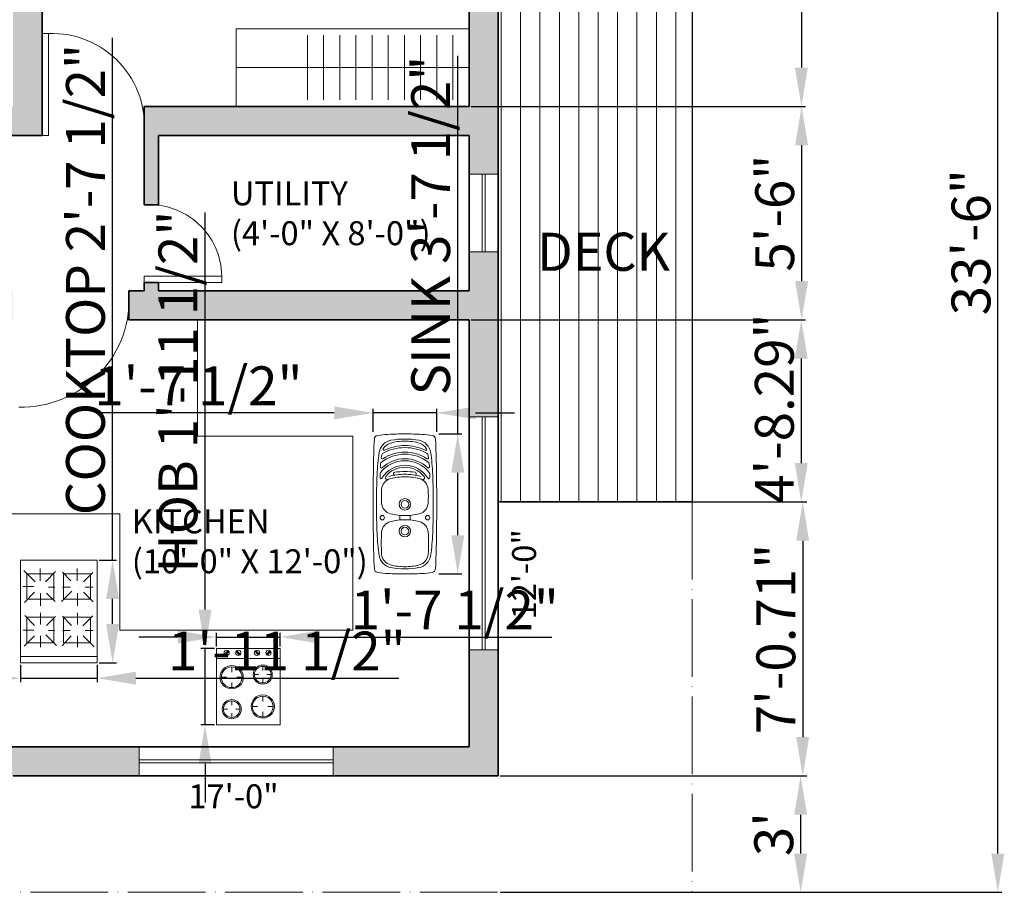
# Model space of a CAD drawing. Units: inches. Extents: x 2364 to 7426, y 1289 to 11972.
# Tile 4 of 6: x 2923 to 3228, y 1362 to 1631. Entities that reach past the tile are written whole.
import ezdxf

# ---------------------------------------------------------------- set-up
doc = ezdxf.new("R2010")
doc.units = ezdxf.units.IN
doc.linetypes.add('ACAD_ISO04W100', pattern=[30, 24, -3, 0, -3])
for name, color, linetype, lineweight in [('A-ANNO-DIMS', 2, 'Continuous', 15), ('A-AREA-IDEN', 7, 'Continuous', 18), ('A-DOOR', 3, 'Continuous', 18), ('A-EQPM', 8, 'Continuous', 18), ('A-FLOR', 7, 'Continuous', 25), ('A-FLOR-CASE', 8, 'Continuous', 18), ('A-FLOR-FIXT', 9, 'Continuous', 18), ('A-FLOR-PATT', 9, 'Continuous', 13), ('A-GLAZ', 4, 'Continuous', 18), ('A-WALL', 7, 'Continuous', 35), ('C-PROP', 3, 'ACAD_ISO04W100', 18)]:
    doc.layers.add(name, color=color, linetype=linetype, lineweight=lineweight)
doc.layers.add('A-WALL-PATT', color=251, linetype='Continuous', lineweight=13, true_color=0x636466)
doc.styles.get("Standard").update_dxf_attribs({"font": 'arial.ttf'})
doc.dimstyles.new('ISO-25', dxfattribs={"dimtxt": 12, "dimasz": 12, "dimexe": 1.25, "dimexo": 0.625, "dimtad": 1, "dimlunit": 3, "dimtxsty": 'Standard', "dimcen": 2.5, "dimadec": 0, "dimazin": 0, "dimtfac": 1, "dimtmove": 0, "dimatfit": 3, "dimfxl": 1, "dimarcsym": 0})

# ---------------------------------------------------------------- blocks, each defined once
blk = doc.blocks.new('A$C16A60262')
at = {"linetype": 'ByBlock'}
for p, q in [((0, 600), (0, 0)), ((487.7, 600), (0, 600)), ((0, 600), (500, 600)), ((0, 600), (500, 600)), ((500, 600), (500, 0)), ((500, 600), (500, 0)), ((500, 520.4), (0, 520.4)), ((119.4, 455.6), (119.4, 414.9)), ((298.2, 394.6), (330.7, 394.6)), ((363.3, 459.6), (363.3, 427.1)), ((428.3, 394.6), (395.8, 394.6)), ((38.1, 374.3), (78.8, 374.3)), ((119.4, 293), (119.4, 333.7)), ((200.7, 374.3), (160.1, 374.3)), ((363.3, 329.6), (363.3, 362.1)), ((119.4, 188.6), (119.4, 156.1)), ((363.3, 225.2), (363.3, 184.6)), ((54.4, 123.6), (86.9, 123.6)), ((119.4, 58.6), (119.4, 91.1)), ((184.4, 123.6), (151.9, 123.6)), ((282, 143.9), (322.6, 143.9)), ((363.3, 62.6), (363.3, 103.3)), ((444.5, 143.9), (403.9, 143.9)), ((0, 0), (500, 0))]:
    blk.add_line(p, q, dxfattribs=at)
for p, q in [((66.2, 557.5), (87.4, 578.7)), ((71.9, 551.8), (66.2, 557.5)), ((93.1, 573), (71.9, 551.8)), ((87.4, 578.7), (93.1, 573)), ((157.6, 572.5), (163.3, 578.1)), ((178.8, 551.2), (157.6, 572.5)), ((163.3, 578.1), (184.5, 556.9)), ((184.5, 556.9), (178.8, 551.2)), ((305.1, 572.5), (310.8, 578.1)), ((326.3, 551.2), (305.1, 572.5)), ((310.8, 578.1), (332, 556.9)), ((332, 556.9), (326.3, 551.2)), ((396.2, 558.5), (417.4, 579.7)), ((401.9, 552.8), (396.2, 558.5)), ((423.1, 574), (401.9, 552.8)), ((417.4, 579.7), (423.1, 574))]:
    blk.add_line(p, q)
for centre in [(80.1, 565.7), (171.2, 565.7), (317.6, 565.7), (408.7, 565.7)]:
    blk.add_circle(centre, 20.6)
for centre, radius in [((119.4, 374.3), 91.3), ((363.3, 394.6), 75), ((119.4, 374.3), 81.3), ((363.3, 394.6), 65), ((363.3, 143.9), 91.3), ((119.4, 123.6), 75), ((119.4, 123.6), 65), ((363.3, 143.9), 81.3)]:
    blk.add_circle(centre, radius, dxfattribs=at)
blk = doc.blocks.new('A$C0AF6382F')
for p, q in [((756, 445), (788, 445)), ((426, 290), (458, 290)), ((426, 210), (458, 210)), ((756, 55), (788, 55))]:
    blk.add_line(p, q)
for centre, radius in [((442, 428), 17.5), ((337, 250), 45), ((337, 250), 30), ((547, 250), 45), ((547, 250), 30), ((442, 72), 17.5)]:
    blk.add_circle(centre, radius)
for centre, radius, start, end in [((752.5, 343.4), 750, 170.67899, 176.94109), ((42, 460), 30, 90, 170.67899), ((245.4, -3004), 3500, 91.51794, 93.33101), ((376.4, -1030.3), 1500, 92.21075, 98.8901), ((550, -14500), 15000, 90, 91.51794), ((550, -5527), 6000, 90, 92.21075), ((550, -14500), 15000, 88.48206, 90), ((550, -5527), 6000, 87.78925, 90), ((723.6, -1030.3), 1500, 81.1099, 87.78925), ((854.6, -3004), 3500, 86.66899, 88.48206), ((1058, 460), 30, 9.32101, 90), ((347.5, 343.4), 750, 3.05891, 9.32101), ((162.2, 339), 114, 98.89008, 169.4341), ((162.2, 339), 94, 94.10767, 165.48561), ((241.4, -764.2), 1200, 85.89233, 94.10767), ((320.7, 339), 94, 14.51439, 85.89233), ((563.3, 339), 94, 94.10767, 165.48561), ((610.5, -766), 1200, 87.42561, 92.57439), ((657.7, 339), 94, 14.51439, 85.89233), ((756, 388.4), 16, 51.02441, 206.67353), ((756, 437), 8, 90, 239.07025), ((644, 250), 210, 0, 59.07025), ((644, 250), 194, 0, 51.02441), ((788, 430), 15, 51.34406, 90), ((644, 250), 245.5, 0, 51.34407), ((839.7, 435.3), 8, 85.01566, 223.44624), ((644, 250), 261.5, 0, 43.44679), ((710, -1051), 1500, 84.0334, 85.01566), ((864.4, 425.9), 15, 38.59821, 84.0334), ((644, 250), 297, 0, 38.59821), ((911.6, 427.3), 8, 82.23571, 213.52556), ((644, 250), 313, 0, 33.52609), ((710, -1051), 1500, 81.38181, 82.23571), ((932.6, 417.2), 15, 30.09023, 81.3818), ((644, 250), 348.5, 0, 30.09022), ((937.8, 339), 114, 10.5659, 81.10992), ((979.1, 412.8), 8, 61.40653, 205.90795), ((644, 250), 364.5, 0, 25.90795), ((938.9, 339), 92, 16.78288, 61.40653), ((2500, 250), 2500, 176.94109, 180), ((640, 250), 600, 169.44537, 190.55463), ((506, 250), 449.1, 165.48561, 180), ((-23.1, 250), 449.1, 0, 14.51439), ((907.1, 250), 449.1, 165.48561, 180), ((313.9, 250), 449.1, 0, 14.51439), ((313.9, 250), 469.1, 0, 15.46747), ((787.6, 328), 11, 189.19758, 189.34977), ((787.6, 328), 11, 9.34978, 137.6835), ((313.9, 250), 491.1, 0, 9.34978), ((644, 250), 400, 0, 16.79873), ((460, 250), 600, 349.44537, 10.55463), ((-1400, 250), 2500, 0, 3.05891), ((2500, 250), 2500, 180, 183.05891), ((506, 250), 449.1, 180, 194.51439), ((-23.1, 250), 449.1, 345.48561, 0), ((907.1, 250), 449.1, 180, 194.51439), ((313.9, 250), 449.1, 345.48561, 0), ((644, 250), 210, 300.92975, 0), ((313.9, 250), 469.1, 344.53253, 0), ((644, 250), 194, 308.97559, 0), ((644, 250), 245.5, 308.65593, 0), ((313.9, 250), 491.1, 350.65022, 0), ((644, 250), 261.5, 316.55321, 0), ((644, 250), 297, 321.40179, 0), ((644, 250), 313, 326.47391, 0), ((644, 250), 348.5, 329.90978, 0), ((644, 250), 364.5, 334.09205, 0), ((644, 250), 400, 343.20127, 0), ((-1400, 250), 2500, 356.94109, 0), ((787.6, 172), 11, 170.65023, 170.80242), ((787.6, 172), 11, 222.3165, 350.65022), ((752.5, 156.6), 750, 183.05891, 189.32101), ((162.2, 161), 114, 190.5659, 261.10992), ((162.2, 161), 94, 194.51439, 265.89233), ((320.7, 161), 94, 274.10767, 345.48561), ((563.3, 161), 94, 194.51439, 265.89233), ((657.7, 161), 94, 274.10767, 345.48561), ((756, 111.6), 16, 153.32647, 308.97559), ((937.8, 161), 114, 278.89008, 349.4341), ((979.1, 87.2), 8, 154.09205, 298.59347), ((938.9, 161), 92, 298.59347, 343.21712), ((347.5, 156.6), 750, 350.67899, 356.94109), ((42, 40), 30, 189.32101, 270), ((245.4, 3504), 3500, 266.66899, 268.48206), ((376.4, 1530.3), 1500, 261.1099, 267.78925), ((550, 15000), 15000, 268.48206, 270), ((241.4, 1264.2), 1200, 265.89233, 274.10767), ((550, 6027), 6000, 267.78925, 270), ((550, 6027), 6000, 270, 272.21075), ((550, 15000), 15000, 270, 271.51794), ((610.5, 1266), 1200, 267.42561, 272.57439), ((756, 63), 8, 120.92975, 270), ((723.6, 1530.3), 1500, 272.21075, 278.8901), ((788, 70), 15, 270, 308.65594), ((839.7, 64.7), 8, 136.55376, 274.98434), ((710, 1551), 1500, 274.98434, 275.9666), ((864.4, 74.1), 15, 275.9666, 321.40179), ((911.6, 72.7), 8, 146.47444, 277.76429), ((710, 1551), 1500, 277.76429, 278.61819), ((932.6, 82.8), 15, 278.6182, 329.90977), ((854.6, 3504), 3500, 271.51794, 273.33101), ((1058, 40), 30, 270, 350.67899)]:
    blk.add_arc(centre, radius, start, end)
blk = doc.blocks.new('A$C114C6ABE')
for p, q in [((0, 0), (0, 806.1)), ((0, 806.1), (602.1, 806.1)), ((602.1, 806.1), (602.1, 0)), ((114.3, 635.6), (26.6, 723.3)), ((50, 699.3), (261.1, 699.3)), ((50, 499.3), (50, 699.3)), ((155.5, 741.3), (155.5, 643.5)), ((195.7, 635.6), (275.8, 715.7)), ((261.1, 699.3), (261.1, 499.3)), ((394.7, 643.5), (330.4, 711.9)), ((338.9, 699.3), (338.9, 499.3)), ((338.9, 699.3), (550, 699.3)), ((444.5, 741.3), (444.5, 643.5)), ((495.3, 635.6), (568.8, 709.1)), ((550, 699.3), (550, 499.3)), ((19.6, 599.3), (104.2, 599.3)), ((110.6, 553.7), (30.2, 473.3)), ((156.6, 545.8), (156.6, 448)), ((205.3, 545.8), (271.3, 479.8)), ((218.5, 594.7), (270.4, 594.7)), ((404.2, 561.7), (323, 480.5)), ((330.3, 594.7), (391, 594.7)), ((446.6, 545.8), (446.6, 448)), ((495.3, 553.7), (570.3, 478.8)), ((508.5, 594.7), (570.4, 594.7)), ((50, 499.3), (261.1, 499.3)), ((338.9, 499.3), (550, 499.3)), ((156.6, 301.3), (156.6, 391.1)), ((446.6, 301.3), (446.6, 391.1)), ((110.6, 293.3), (33.5, 370.5)), ((50, 156.9), (50, 356.9)), ((261.1, 356.9), (50, 356.9)), ((205.3, 293.3), (275.4, 363.4)), ((261.1, 356.9), (261.1, 156.9)), ((401.1, 293.3), (329.5, 364.9)), ((550, 356.9), (338.9, 356.9)), ((338.9, 356.9), (338.9, 156.9)), ((489.7, 291), (567.7, 369)), ((550, 356.9), (550, 156.9)), ((104.2, 256.9), (19.6, 256.9)), ((218.5, 252.4), (270.4, 252.4)), ((330.3, 252.4), (391, 252.4)), ((508.5, 252.4), (570.4, 252.4)), ((110.6, 211.5), (30, 130.8)), ((261.1, 156.9), (50, 156.9)), ((156.6, 211.5), (156.6, 121.7)), ((198.9, 219.4), (282.7, 135.7)), ((397.9, 211.5), (326.4, 131.6)), ((550, 156.9), (338.9, 156.9)), ((446.6, 211.5), (446.6, 121.7)), ((492.1, 211.5), (579, 124.6)), ((602.1, 50), (0, 50)), ((602.1, 0), (0, 0))]:
    blk.add_line(p, q)
blk = doc.blocks.new('*D20')
at = {"layer": 'A-ANNO-DIMS', "color": 0, "lineweight": -2, "transparency": 16777216}
for p, q in [((3071.73, 1763.54), (3166.08, 1763.54)), ((3164.83, 1751.54), (3164.83, 1616.54)), ((3062.73, 1604.54), (3166.08, 1604.54))]:
    blk.add_line(p, q, dxfattribs=at)
at = {"layer": 'A-ANNO-DIMS', "color": 0, "lineweight": 100, "transparency": 16777216}
for points in [[(3162.83, 1751.54), (3166.83, 1751.54), (3164.83, 1763.54)], [(3162.83, 1616.54), (3166.83, 1616.54), (3164.83, 1604.54)]]:
    blk.add_solid(points, dxfattribs=at)
at = {"layer": 'Defpoints', "color": 0, "lineweight": 100, "transparency": 16777216}
for p in [(3071.1, 1763.54), (3062.1, 1604.54), (3164.83, 1604.54)]:
    blk.add_point(p, dxfattribs=at)
at = {"layer": 'A-ANNO-DIMS', "color": 0, "transparency": 16777216, "insert": (3158.08, 1684.04), "char_height": 12, "attachment_point": 5, "rotation": 90}
blk.add_mtext('13\'-3"', dxfattribs=at)
blk = doc.blocks.new('*D21')
at = {"layer": 'A-ANNO-DIMS', "color": 0, "lineweight": -2, "transparency": 16777216}
for p, q in [((3071.73, 1604.54), (3166.14, 1604.54)), ((3164.89, 1592.54), (3164.89, 1550.54)), ((3062.73, 1538.54), (3166.14, 1538.54))]:
    blk.add_line(p, q, dxfattribs=at)
at = {"layer": 'A-ANNO-DIMS', "color": 0, "lineweight": 100, "transparency": 16777216}
for points in [[(3162.89, 1592.54), (3166.89, 1592.54), (3164.89, 1604.54)], [(3162.89, 1550.54), (3166.89, 1550.54), (3164.89, 1538.54)]]:
    blk.add_solid(points, dxfattribs=at)
at = {"layer": 'Defpoints', "color": 0, "lineweight": 100, "transparency": 16777216}
for p in [(3071.1, 1604.54), (3062.1, 1538.54), (3164.89, 1538.54)]:
    blk.add_point(p, dxfattribs=at)
at = {"layer": 'A-ANNO-DIMS', "color": 0, "transparency": 16777216, "insert": (3158.13, 1571.54), "char_height": 12, "attachment_point": 5, "rotation": 90}
blk.add_mtext('5\'-6"', dxfattribs=at)
blk = doc.blocks.new('*D22')
at = {"layer": 'A-ANNO-DIMS', "color": 0, "lineweight": -2, "transparency": 16777216}
for p, q in [((3062.73, 1538.54), (3166.04, 1538.54)), ((3164.79, 1526.54), (3164.79, 1494.25)), ((3071.73, 1482.25), (3166.04, 1482.25))]:
    blk.add_line(p, q, dxfattribs=at)
at = {"layer": 'A-ANNO-DIMS', "color": 0, "lineweight": 100, "transparency": 16777216}
for points in [[(3162.79, 1526.54), (3166.79, 1526.54), (3164.79, 1538.54)], [(3162.79, 1494.25), (3166.79, 1494.25), (3164.79, 1482.25)]]:
    blk.add_solid(points, dxfattribs=at)
at = {"layer": 'Defpoints', "color": 0, "lineweight": 100, "transparency": 16777216}
for p in [(3062.1, 1538.54), (3071.1, 1482.25), (3164.79, 1482.25)]:
    blk.add_point(p, dxfattribs=at)
at = {"layer": 'A-ANNO-DIMS', "color": 0, "transparency": 16777216, "insert": (3158.03, 1511.09), "char_height": 12, "attachment_point": 5, "rotation": 90}
blk.add_mtext('4\'-8.29"', dxfattribs=at)
blk = doc.blocks.new('*D23')
at = {"layer": 'A-ANNO-DIMS', "color": 0, "lineweight": -2, "transparency": 16777216}
for p, q in [((3071.73, 1482.25), (3166.49, 1482.25)), ((3165.24, 1470.25), (3165.24, 1409.54)), ((3071.73, 1397.54), (3166.49, 1397.54))]:
    blk.add_line(p, q, dxfattribs=at)
at = {"layer": 'A-ANNO-DIMS', "color": 0, "lineweight": 100, "transparency": 16777216}
for points in [[(3163.24, 1470.25), (3167.24, 1470.25), (3165.24, 1482.25)], [(3163.24, 1409.54), (3167.24, 1409.54), (3165.24, 1397.54)]]:
    blk.add_solid(points, dxfattribs=at)
at = {"layer": 'Defpoints', "color": 0, "lineweight": 100, "transparency": 16777216}
for p in [(3071.1, 1482.25), (3071.1, 1397.54), (3165.24, 1397.54)]:
    blk.add_point(p, dxfattribs=at)
at = {"layer": 'A-ANNO-DIMS', "color": 0, "transparency": 16777216, "insert": (3158.49, 1439.9), "char_height": 12, "attachment_point": 5, "rotation": 90}
blk.add_mtext('7\'-0.71"', dxfattribs=at)
blk = doc.blocks.new('*D24')
at = {"layer": 'A-ANNO-DIMS', "color": 0, "lineweight": -2, "transparency": 16777216}
for p, q in [((3071.73, 1397.54), (3165.85, 1397.54)), ((3164.6, 1385.54), (3164.6, 1373.54)), ((3071.73, 1361.54), (3165.85, 1361.54))]:
    blk.add_line(p, q, dxfattribs=at)
at = {"layer": 'A-ANNO-DIMS', "color": 0, "lineweight": 100, "transparency": 16777216}
for points in [[(3162.6, 1385.54), (3166.6, 1385.54), (3164.6, 1397.54)], [(3162.6, 1373.54), (3166.6, 1373.54), (3164.6, 1361.54)]]:
    blk.add_solid(points, dxfattribs=at)
at = {"layer": 'Defpoints', "color": 0, "lineweight": 100, "transparency": 16777216}
for p in [(3071.1, 1397.54), (3071.1, 1361.54), (3164.6, 1361.54)]:
    blk.add_point(p, dxfattribs=at)
at = {"layer": 'A-ANNO-DIMS', "color": 0, "transparency": 16777216, "insert": (3157.84, 1379.54), "char_height": 12, "attachment_point": 5, "rotation": 90}
blk.add_mtext("3'", dxfattribs=at)
blk = doc.blocks.new('*D25')
at = {"layer": 'A-ANNO-DIMS', "color": 0, "lineweight": -2, "transparency": 16777216}
for p, q in [((3131.73, 1763.54), (3226.82, 1763.54)), ((3225.57, 1373.54), (3225.57, 1751.54)), ((3131.73, 1361.54), (3226.82, 1361.54))]:
    blk.add_line(p, q, dxfattribs=at)
at = {"layer": 'A-ANNO-DIMS', "color": 0, "lineweight": 100, "transparency": 16777216}
for points in [[(3223.57, 1751.54), (3227.57, 1751.54), (3225.57, 1763.54)], [(3223.57, 1373.54), (3227.57, 1373.54), (3225.57, 1361.54)]]:
    blk.add_solid(points, dxfattribs=at)
at = {"layer": 'Defpoints', "color": 0, "lineweight": 100, "transparency": 16777216}
for p in [(3131.1, 1763.54), (3225.57, 1763.54), (3131.1, 1361.54)]:
    blk.add_point(p, dxfattribs=at)
at = {"layer": 'A-ANNO-DIMS', "color": 0, "transparency": 16777216, "insert": (3218.81, 1562.54), "char_height": 12, "attachment_point": 5, "rotation": 90}
blk.add_mtext('33\'-6"', dxfattribs=at)
blk = doc.blocks.new('WIN-72IN')
for p, q in [((0, 0), (0, 9)), ((72, 0), (72, 9)), ((72, 5), (0, 5)), ((72, 4), (0, 4))]:
    blk.add_line(p, q)
blk = doc.blocks.new('WIN-24IN')
for p, q in [((0, 0), (0, 9)), ((24, 0), (24, 9)), ((0, 5), (24, 5)), ((0, 4), (24, 4))]:
    blk.add_line(p, q)
blk = doc.blocks.new('*D47')
at = {"layer": 'A-ANNO-DIMS', "color": 0, "lineweight": -2, "transparency": 16777216}
for p, q in [((2980.45, 1448.93), (2980.45, 1571.7)), ((2983.37, 1436.93), (2979.2, 1436.93)), ((2980.45, 1413.31), (2980.45, 1436.93)), ((2983.37, 1413.31), (2979.2, 1413.31)), ((2980.45, 1401.31), (2980.45, 1389.31))]:
    blk.add_line(p, q, dxfattribs=at)
at = {"layer": 'A-ANNO-DIMS', "color": 0, "lineweight": 100, "transparency": 16777216}
for points in [[(2978.45, 1448.93), (2982.45, 1448.93), (2980.45, 1436.93)], [(2978.45, 1401.31), (2982.45, 1401.31), (2980.45, 1413.31)]]:
    blk.add_solid(points, dxfattribs=at)
at = {"layer": 'Defpoints', "color": 0, "lineweight": 100, "transparency": 16777216}
for p in [(2980.45, 1436.93), (2984, 1436.93), (2984, 1413.31)]:
    blk.add_point(p, dxfattribs=at)
at = {"layer": 'A-ANNO-DIMS', "color": 0, "transparency": 16777216, "insert": (2973.62, 1516.32), "char_height": 12, "attachment_point": 5, "rotation": 90}
blk.add_mtext('HOB 1\'-11 1/2"', dxfattribs=at)
blk = doc.blocks.new('*D48')
at = {"layer": 'A-ANNO-DIMS', "color": 0, "lineweight": -2, "transparency": 16777216}
for p, q in [((2972, 1440.47), (2960, 1440.47)), ((2984, 1437.55), (2984, 1441.72)), ((2984, 1440.47), (3003.68, 1440.47)), ((3003.68, 1437.55), (3003.68, 1441.72)), ((3015.68, 1440.47), (3087.66, 1440.47))]:
    blk.add_line(p, q, dxfattribs=at)
at = {"layer": 'A-ANNO-DIMS', "color": 0, "lineweight": 100, "transparency": 16777216}
for points in [[(2972, 1442.47), (2972, 1438.47), (2984, 1440.47)], [(3015.68, 1442.47), (3015.68, 1438.47), (3003.68, 1440.47)]]:
    blk.add_solid(points, dxfattribs=at)
at = {"layer": 'Defpoints', "color": 0, "lineweight": 100, "transparency": 16777216}
for p in [(3003.68, 1440.47), (2984, 1436.93), (3003.68, 1436.93)]:
    blk.add_point(p, dxfattribs=at)
at = {"layer": 'A-ANNO-DIMS', "color": 0, "transparency": 16777216, "insert": (3057.67, 1447.3), "char_height": 12, "attachment_point": 5}
blk.add_mtext('1\'-7 1/2"', dxfattribs=at)
blk = doc.blocks.new('*D49')
at = {"layer": 'A-ANNO-DIMS', "color": 0, "lineweight": -2, "transparency": 16777216}
for p, q in [((3058.59, 1503.27), (3058.59, 1620.11)), ((3052.72, 1503.27), (3059.84, 1503.27)), ((3058.59, 1471.96), (3058.59, 1491.27)), ((3052.72, 1459.96), (3059.84, 1459.96))]:
    blk.add_line(p, q, dxfattribs=at)
at = {"layer": 'A-ANNO-DIMS', "color": 0, "lineweight": 100, "transparency": 16777216}
for points in [[(3056.59, 1491.27), (3060.59, 1491.27), (3058.59, 1503.27)], [(3056.59, 1471.96), (3060.59, 1471.96), (3058.59, 1459.96)]]:
    blk.add_solid(points, dxfattribs=at)
at = {"layer": 'Defpoints', "color": 0, "lineweight": 100, "transparency": 16777216}
for p in [(3052.09, 1503.27), (3058.59, 1503.27), (3052.09, 1459.96)]:
    blk.add_point(p, dxfattribs=at)
at = {"layer": 'A-ANNO-DIMS', "color": 0, "transparency": 16777216, "insert": (3051.76, 1567.69), "char_height": 12, "attachment_point": 5, "rotation": 90}
blk.add_mtext('SINK 3\'-7 1/2"', dxfattribs=at)
blk = doc.blocks.new('*D50')
at = {"layer": 'A-ANNO-DIMS', "color": 0, "lineweight": -2, "transparency": 16777216}
for p, q in [((3032.41, 1503.89), (3032.41, 1511.01)), ((3052.09, 1503.89), (3052.09, 1511.01)), ((3020.41, 1509.76), (2948.43, 1509.76)), ((3052.09, 1509.76), (3032.41, 1509.76)), ((3064.09, 1509.76), (3076.09, 1509.76))]:
    blk.add_line(p, q, dxfattribs=at)
at = {"layer": 'A-ANNO-DIMS', "color": 0, "lineweight": 100, "transparency": 16777216}
for points in [[(3020.41, 1511.76), (3020.41, 1507.76), (3032.41, 1509.76)], [(3064.09, 1511.76), (3064.09, 1507.76), (3052.09, 1509.76)]]:
    blk.add_solid(points, dxfattribs=at)
at = {"layer": 'Defpoints', "color": 0, "lineweight": 100, "transparency": 16777216}
for p in [(3032.41, 1509.76), (3032.41, 1503.27), (3052.09, 1503.27)]:
    blk.add_point(p, dxfattribs=at)
at = {"layer": 'A-ANNO-DIMS', "color": 0, "transparency": 16777216, "insert": (2978.42, 1516.59), "char_height": 12, "attachment_point": 5}
blk.add_mtext('1\'-7 1/2"', dxfattribs=at)
blk = doc.blocks.new('*D51')
at = {"layer": 'A-ANNO-DIMS', "color": 0, "lineweight": -2, "transparency": 16777216}
for p, q in [((2951.87, 1464.26), (2951.87, 1625.72)), ((2947.73, 1464.26), (2953.12, 1464.26)), ((2951.87, 1444.52), (2951.87, 1452.26)), ((2947.73, 1432.52), (2953.12, 1432.52))]:
    blk.add_line(p, q, dxfattribs=at)
at = {"layer": 'A-ANNO-DIMS', "color": 0, "lineweight": 100, "transparency": 16777216}
for points in [[(2949.87, 1452.26), (2953.87, 1452.26), (2951.87, 1464.26)], [(2949.87, 1444.52), (2953.87, 1444.52), (2951.87, 1432.52)]]:
    blk.add_solid(points, dxfattribs=at)
at = {"layer": 'Defpoints', "color": 0, "lineweight": 100, "transparency": 16777216}
for p in [(2947.11, 1464.26), (2951.87, 1464.26), (2947.11, 1432.52)]:
    blk.add_point(p, dxfattribs=at)
at = {"layer": 'A-ANNO-DIMS', "color": 0, "transparency": 16777216, "insert": (2945.04, 1550.99), "char_height": 12, "attachment_point": 5, "rotation": 90}
blk.add_mtext('COOKTOP 2\'-7 1/2"', dxfattribs=at)
blk = doc.blocks.new('*D52')
at = {"layer": 'A-ANNO-DIMS', "color": 0, "lineweight": -2, "transparency": 16777216}
for p, q in [((2923.4, 1431.9), (2923.4, 1426.51)), ((2947.11, 1431.9), (2947.11, 1426.51)), ((2911.4, 1427.76), (2899.4, 1427.76)), ((2923.4, 1427.76), (2947.11, 1427.76)), ((2959.11, 1427.76), (3040.41, 1427.76))]:
    blk.add_line(p, q, dxfattribs=at)
at = {"layer": 'A-ANNO-DIMS', "color": 0, "lineweight": 100, "transparency": 16777216}
for points in [[(2911.4, 1429.76), (2911.4, 1425.76), (2923.4, 1427.76)], [(2959.11, 1429.76), (2959.11, 1425.76), (2947.11, 1427.76)]]:
    blk.add_solid(points, dxfattribs=at)
at = {"layer": 'Defpoints', "color": 0, "lineweight": 100, "transparency": 16777216}
for p in [(2923.4, 1432.52), (2947.11, 1432.52), (2947.11, 1427.76)]:
    blk.add_point(p, dxfattribs=at)
at = {"layer": 'A-ANNO-DIMS', "color": 0, "transparency": 16777216, "insert": (3005.76, 1434.59), "char_height": 12, "attachment_point": 5}
blk.add_mtext('1\'-11 1/2"', dxfattribs=at)

msp = doc.modelspace()

# ---------------------------------------------------------------- hatches: boundary and pattern name
at = {"layer": 'A-FLOR-PATT'}
h = msp.add_hatch(dxfattribs=at)
h.set_pattern_fill('ANSI31', color=256, scale=1.889764, angle=45, style=0)
h.paths.add_polyline_path([(3071.103, 1482.254), (3131.103, 1482.254), (3131.103, 1643.544), (3071.103, 1643.544)])
at = {"layer": 'A-WALL-PATT'}
h = msp.add_hatch(color=256, dxfattribs=at)
h.dxf.hatch_style = 1
h.paths.add_polyline_path([(2522.103, 1763.544), (2477.103, 1763.544), (2477.103, 1646.544), (2486.103, 1646.544), (2486.103, 1754.544), (2522.103, 1754.544)])
h.paths.add_polyline_path([(2657.103, 1763.544), (2594.103, 1763.544), (2594.103, 1754.544), (2630.103, 1754.544), (2630.103, 1625.388), (2632.457, 1625.388, -0.0509344), (2639.103, 1625.388), (2639.103, 1654.044), (2640.627, 1654.044), (2640.627, 1658.544), (2639.103, 1658.544), (2639.103, 1754.544), (2657.103, 1754.544)])
h.paths.add_polyline_path([(2746.353, 1763.544), (2681.103, 1763.544), (2681.103, 1754.544), (2699.103, 1754.544), (2699.103, 1658.544), (2670.627, 1658.544), (2670.627, 1656.552, -0.0218135), (2670.627, 1654.044), (2699.103, 1654.044), (2699.103, 1595.544), (2820.603, 1595.544, -0.0518861), (2820.603, 1602.304), (2820.603, 1604.544), (2708.103, 1604.544), (2708.103, 1754.544), (2746.353, 1754.544)])
h.paths.add_polyline_path([(2879.103, 1763.544), (2818.353, 1763.544), (2818.353, 1754.544), (2856.603, 1754.544), (2856.603, 1666.044), (2921.103, 1666.044), (2921.103, 1604.544), (2897.103, 1604.544), (2897.103, 1595.544), (2930.103, 1595.544), (2930.103, 1627.044), (2930.103, 1754.544), (3062.103, 1754.544), (3062.103, 1715.544), (3071.103, 1715.544), (3071.103, 1763.544), (2903.103, 1763.544), (2903.103, 1754.544), (2921.103, 1754.544), (2921.103, 1670.544), (2861.103, 1670.544), (2861.103, 1754.544), (2879.103, 1754.544)])
h.paths.add_polyline_path([(3071.103, 1643.544), (3062.103, 1643.544), (3062.103, 1604.544), (2961.603, 1604.544), (2961.603, 1601.334, -0.0507006), (2961.603, 1595.544), (2961.603, 1574.085, -0.036481), (2964.864, 1574.085), (2966.103, 1574.085), (2966.103, 1595.544), (3062.103, 1595.544), (3062.103, 1583.544), (3071.103, 1583.544)])
h.paths.add_polyline_path([(3071.103, 1559.544), (3062.103, 1559.544), (3062.103, 1547.544), (2966.103, 1547.544), (2966.103, 1550.085), (2961.603, 1550.085), (2961.603, 1547.544), (2956.9, 1547.544, -0.039283), (2956.9, 1542.306), (2956.9, 1538.544), (3062.103, 1538.544), (3062.103, 1508.544), (3071.103, 1508.544)])
h.paths.add_polyline_path([(3071.103, 1436.544), (3062.103, 1436.544), (3062.103, 1406.544), (3020.103, 1406.544), (3020.103, 1397.544), (3071.103, 1397.544)])
h.paths.add_polyline_path([(2960.103, 1406.544), (2918.103, 1406.544), (2918.103, 1538.544), (2920.9, 1538.544), (2920.9, 1547.544), (2909.103, 1547.544), (2909.103, 1406.544), (2875.194, 1406.544), (2875.194, 1397.544), (2921.103, 1397.544), (2960.103, 1397.544)])
h.paths.add_polyline_path([(2803.194, 1406.544), (2739.149, 1406.544), (2739.149, 1397.544), (2803.194, 1397.544)])
h.paths.add_polyline_path([(2667.149, 1406.544), (2603.103, 1406.544), (2603.103, 1435.657), (2594.103, 1435.657), (2594.103, 1397.544), (2667.149, 1397.544)])
h.paths.add_polyline_path([(2603.103, 1536.771), (2600.612, 1536.771, -0.0497705), (2594.103, 1536.771), (2594.103, 1507.657), (2603.103, 1507.657)])
h.paths.add_polyline_path([(2639.103, 1589.388), (2630.103, 1589.388), (2630.103, 1586.544), (2486.103, 1586.544), (2486.103, 1610.544), (2477.103, 1610.544), (2477.103, 1577.544), (2594.103, 1577.544), (2594.103, 1572.771), (2603.103, 1572.771), (2603.103, 1577.544), (2639.103, 1577.544)])
h.paths.add_polyline_path([(2636.627, 1719.186), (2701.024, 1719.186), (2701.024, 1746.896), (2636.627, 1746.896)], flags=9)

# ---------------------------------------------------------------- linework, layer by layer
at = {"layer": 'A-DOOR'}
for p, q in [((2930.103, 1595.544), (2930.103, 1627.044)), ((2930.103, 1627.044), (2932.103, 1627.044)), ((2932.103, 1627.044), (2932.103, 1595.544)), ((2932.103, 1595.544), (2930.103, 1595.544)), ((2985.603, 1552.085), (2961.603, 1552.085)), ((2961.603, 1552.085), (2961.603, 1550.085)), ((2961.603, 1550.085), (2985.603, 1550.085)), ((2985.603, 1550.085), (2985.603, 1552.085))]:
    msp.add_line(p, q, dxfattribs=at)
for centre, radius, start, end in [((2933.127, 1598.439), 28.623, 354.19511, 92.04914), ((2963.234, 1551.772), 22.372, 0.80055, 94.17856), ((2923.614, 1544.925), 33.388, 268.77397, 4.49919)]:
    msp.add_arc(centre, radius, start, end, dxfattribs=at)
at = {"layer": 'A-FLOR'}
for p, q in [((3131.103, 1643.544), (3131.103, 1482.254)), ((3131.103, 1482.254), (3071.103, 1482.254))]:
    msp.add_line(p, q, dxfattribs=at)
at = {"layer": 'A-FLOR-CASE'}
for p, q in [((2990.103, 1628.544), (3062.103, 1628.544)), ((2990.103, 1604.544), (2990.103, 1628.544)), ((3012.103, 1606.544), (3012.103, 1626.544)), ((3017.103, 1606.544), (3017.103, 1626.544)), ((3022.103, 1606.544), (3022.103, 1626.544)), ((3027.103, 1606.544), (3027.103, 1626.544)), ((3032.103, 1606.544), (3032.103, 1626.544)), ((3037.103, 1606.544), (3037.103, 1626.544)), ((3042.103, 1606.544), (3042.103, 1626.544)), ((3047.103, 1606.544), (3047.103, 1626.544)), ((3052.103, 1606.544), (3052.103, 1626.544)), ((3057.103, 1606.544), (3057.103, 1626.544)), ((2990.103, 1616.544), (3062.103, 1616.544)), ((2978.103, 1502.544), (2978.103, 1538.544)), ((2978.103, 1502.544), (3026.103, 1502.544)), ((3026.103, 1442.544), (3026.103, 1502.544)), ((2954.103, 1478.544), (2918.103, 1478.544)), ((2954.103, 1442.544), (2954.103, 1478.544)), ((2954.103, 1442.544), (3026.103, 1442.544))]:
    msp.add_line(p, q, dxfattribs=at)
at = {"layer": 'A-GLAZ'}
for p, q in [((2960.103, 1406.544), (2960.103, 1397.544)), ((3020.103, 1406.544), (3020.103, 1397.544)), ((2960.103, 1402.544), (3020.103, 1402.544)), ((2960.103, 1401.544), (3020.103, 1401.544))]:
    msp.add_line(p, q, dxfattribs=at)
at = {"layer": 'A-WALL'}
for p, q in [((3071.103, 1397.544), (3071.103, 1763.544)), ((2930.103, 1604.544), (2930.103, 1754.544)), ((2930.103, 1604.544), (2930.103, 1754.544)), ((3062.103, 1604.544), (3062.103, 1754.544)), ((3062.103, 1604.544), (3062.103, 1754.544)), ((2930.103, 1604.544), (2930.103, 1595.544)), ((2961.603, 1604.544), (3062.103, 1604.544)), ((2961.603, 1595.544), (2961.603, 1604.544)), ((2897.103, 1595.544), (2930.103, 1595.544)), ((2961.603, 1574.085), (2961.603, 1595.544)), ((2966.103, 1595.544), (3062.103, 1595.544)), ((2966.103, 1574.085), (2966.103, 1595.544)), ((3062.103, 1547.544), (3062.103, 1595.544)), ((2961.603, 1574.085), (2966.103, 1574.085)), ((2961.603, 1547.544), (2961.603, 1550.085)), ((2961.603, 1550.085), (2966.103, 1550.085)), ((2966.103, 1547.544), (2966.103, 1550.085)), ((2956.9, 1538.544), (2956.9, 1547.544)), ((2956.9, 1547.544), (2961.603, 1547.544)), ((2966.103, 1547.544), (3062.103, 1547.544)), ((2956.9, 1538.544), (3062.103, 1538.544)), ((3062.103, 1406.544), (3062.103, 1538.544)), ((2918.103, 1406.544), (3062.103, 1406.544)), ((2921.103, 1397.544), (3071.103, 1397.544))]:
    msp.add_line(p, q, dxfattribs=at)
at = {"layer": 'C-PROP'}
for p, q in [((3131.103, 1482.254), (3131.103, 1361.544)), ((3131.103, 1361.544), (2921.103, 1361.544))]:
    msp.add_line(p, q, dxfattribs=at)

# ---------------------------------------------------------------- block references
at = {"layer": 'A-EQPM', "xscale": 0.0393700787401575, "yscale": 0.0393700787401575, "zscale": 0.0393700787401575}
for name, p in [('A$C114C6ABE', (2923.405, 1432.522)), ('A$C16A60262', (2983.998, 1413.308))]:
    msp.add_blockref(name, p, dxfattribs=at)
at = {"layer": 'A-FLOR-FIXT', "xscale": 0.0393700787401575, "yscale": 0.0393700787401575, "zscale": 0.0393700787401575, "rotation": 90}
msp.add_blockref('A$C0AF6382F', (3052.093, 1459.961), dxfattribs=at)
at = {"layer": 'A-GLAZ'}
for name, p, rotation in [('WIN-24IN', (3062.103, 1583.544), 270.0000000000007), ('WIN-72IN', (3062.103, 1508.544), 270)]:
    msp.add_blockref(name, p, dxfattribs=dict(at, rotation=rotation))

# ---------------------------------------------------------------- texts
at = {"layer": 'A-ANNO-DIMS', "insert": (3075.395, 1445.923), "char_height": 7.4003, "attachment_point": 1, "rotation": 90}
msp.add_mtext_dynamic_manual_height_columns('12\'-0"', width=192.6715, gutter_width=37.001, heights=[0], dxfattribs=at)
at = {"layer": 'A-ANNO-DIMS', "insert": (2975.307, 1394.936), "char_height": 7.4003, "attachment_point": 1}
msp.add_mtext_dynamic_manual_height_columns('17\'-0"', width=192.6715, gutter_width=37.001, heights=[0], dxfattribs=at)
at = {"layer": 'A-AREA-IDEN', "attachment_point": 1}
for s, width, gutter_width, insert, char_height in [('UTILITY \\P(4\'-0" X 8\'-0")', 192.6715, 37.001, (2988.451, 1581.359), 7.40027), ('DECK ', 306.54224, 58.869, (3083.103, 1565.467), 11.7739), ('KITCHEN \\P(10\'-0" X 12\'-0")', 192.6715, 37.001, (2957.823, 1479.931), 7.40027)]:
    msp.add_mtext_dynamic_manual_height_columns(s, width=width, gutter_width=gutter_width, heights=[0], dxfattribs=dict(at, insert=insert, char_height=char_height))

# ---------------------------------------------------------------- dimensions: what is measured, and where the dimension line sits
at = {"layer": 'A-ANNO-DIMS'}
for base, p1, p2, angle, override, picture, middle in [((3164.833, 1604.544), (3071.103, 1763.544), (3062.103, 1604.544), 90, {"dimclrd": 0, "dimclre": 0, "dimclrt": 0}, '*D20', (3158.077, 1684.044)), ((3225.565, 1763.544), (3131.103, 1361.544), (3131.103, 1763.544), 90, {"dimclrd": 0, "dimclre": 0, "dimclrt": 0}, '*D25', (3218.809, 1562.544)), ((3164.886, 1538.544), (3071.103, 1604.544), (3062.103, 1538.544), 90, {"dimclrd": 0, "dimclre": 0, "dimclrt": 0}, '*D21', (3158.134, 1571.544)), ((3032.408, 1509.764), (3052.093, 1503.268), (3032.408, 1503.268), 180, {"dimdec": 1, "dimlfac": 1, "dimrnd": 0, "dimzin": 1, "dimdsep": 46, "dimlunit": 4, "dimfrac": 2}, '*D50', (2978.417, 1516.594)), ((3165.24, 1397.544), (3071.103, 1482.254), (3071.103, 1397.544), 90, {"dimclrd": 0, "dimclre": 0, "dimclrt": 0}, '*D23', (3158.488, 1439.899)), ((3164.598, 1361.544), (3071.103, 1397.544), (3071.103, 1361.544), 90, {"dimclrd": 0, "dimclre": 0, "dimclrt": 0}, '*D24', (3157.842, 1379.544))]:
    dim = msp.add_linear_dim(base=base, p1=p1, p2=p2, angle=angle, dimstyle='ISO-25', override=override, dxfattribs=at)
    dim.commit()
    dim.dimension.update_dxf_attribs({"geometry": picture, "text_midpoint": middle})
for base, p1, p2, text, picture, middle in [((2951.87, 1464.259), (2947.11, 1432.522), (2947.11, 1464.259), 'COOKTOP <>', '*D51', (2945.037, 1550.988)), ((3058.589, 1503.268), (3052.093, 1459.961), (3052.093, 1503.268), 'SINK <>', '*D49', (3051.755, 1567.687)), ((2980.454, 1436.93), (2983.998, 1413.308), (2983.998, 1436.93), 'HOB <>', '*D47', (2973.621, 1516.316))]:
    dim = msp.add_linear_dim(base=base, p1=p1, p2=p2, angle=90, text=text, dimstyle='ISO-25', override={"dimdec": 1, "dimlfac": 1, "dimrnd": 0, "dimzin": 1, "dimdsep": 46, "dimlunit": 4, "dimfrac": 2}, dxfattribs=at)
    dim.commit()
    dim.dimension.update_dxf_attribs({"geometry": picture, "text_midpoint": middle})
dim = msp.add_linear_dim(base=(3164.786, 1482.254), p1=(3062.103, 1538.544), p2=(3071.103, 1482.254), angle=90, dimstyle='ISO-25', override={"dimclrd": 0, "dimclre": 0, "dimclrt": 0}, dxfattribs=at)
dim.commit()
dim.dimension.update_dxf_attribs({"geometry": '*D22', "text_midpoint": (3164.786, 1511.094), "dimtype": 160})
for base, p1, p2, picture, middle in [((3003.683, 1440.473), (2983.998, 1436.93), (3003.683, 1436.93), '*D48', (3057.673, 1447.303)), ((2947.11, 1427.761), (2923.405, 1432.522), (2947.11, 1432.522), '*D52', (3005.762, 1434.591))]:
    dim = msp.add_linear_dim(base=base, p1=p1, p2=p2, dimstyle='ISO-25', override={"dimdec": 1, "dimlfac": 1, "dimrnd": 0, "dimzin": 1, "dimdsep": 46, "dimlunit": 4, "dimfrac": 2}, dxfattribs=at)
    dim.commit()
    dim.dimension.update_dxf_attribs({"geometry": picture, "text_midpoint": middle})

doc.saveas('drawing.dxf')
